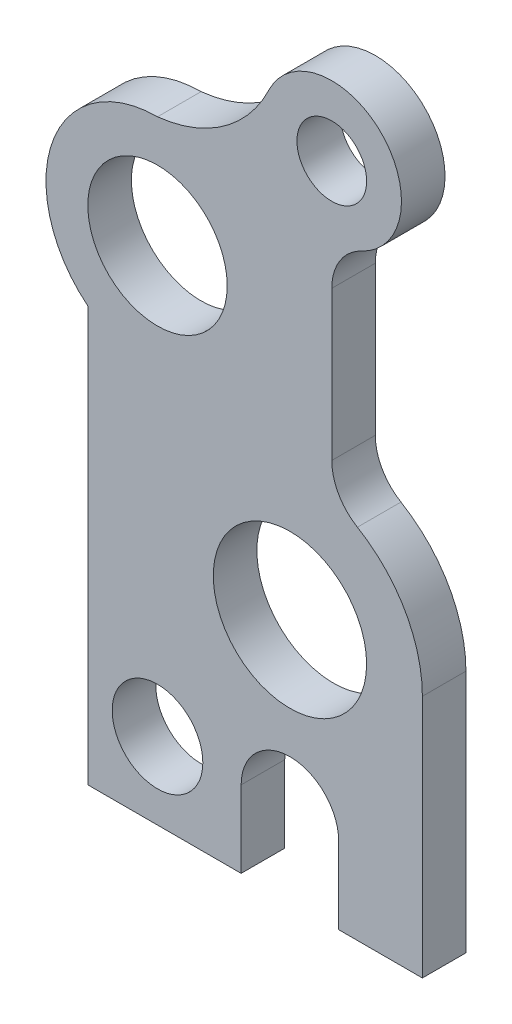
ISO-10303-21;
HEADER;
FILE_DESCRIPTION(('STEP AP214'),'2;1');
FILE_NAME('part.step','',(''),(''),'','','');
FILE_SCHEMA(('AUTOMOTIVE_DESIGN { 1 0 10303 214 1 1 1 1 }'));
ENDSEC;
DATA;
#1=APPLICATION_CONTEXT('core data for automotive mechanical design processes');
#2=APPLICATION_PROTOCOL_DEFINITION('international standard','automotive_design',2000,#1);
#3=PRODUCT_CONTEXT('',#1,'mechanical');
#4=PRODUCT('Part','Part','',(#3));
#5=PRODUCT_RELATED_PRODUCT_CATEGORY('part','',(#4));
#6=PRODUCT_DEFINITION_FORMATION('','',#4);
#7=PRODUCT_DEFINITION_CONTEXT('part definition',#1,'design');
#8=PRODUCT_DEFINITION('design','',#6,#7);
#9=PRODUCT_DEFINITION_SHAPE('','',#8);
#10=(LENGTH_UNIT() NAMED_UNIT(*) SI_UNIT(.MILLI.,.METRE.));
#11=(NAMED_UNIT(*) PLANE_ANGLE_UNIT() SI_UNIT($,.RADIAN.));
#12=(NAMED_UNIT(*) SI_UNIT($,.STERADIAN.) SOLID_ANGLE_UNIT());
#13=UNCERTAINTY_MEASURE_WITH_UNIT(LENGTH_MEASURE(1.E-05),#10,'distance_accuracy_value','');
#14=(GEOMETRIC_REPRESENTATION_CONTEXT(3) GLOBAL_UNCERTAINTY_ASSIGNED_CONTEXT((#13)) GLOBAL_UNIT_ASSIGNED_CONTEXT((#10,
#11,#12)) REPRESENTATION_CONTEXT('',''));
#15=CARTESIAN_POINT('',(0.,0.,0.));
#16=DIRECTION('',(0.,0.,1.));
#17=DIRECTION('',(1.,0.,0.));
#18=AXIS2_PLACEMENT_3D('',#15,#16,#17);
#19=CARTESIAN_POINT('',(96.,0.,12.5));
#20=DIRECTION('',(-1.,0.,0.));
#21=DIRECTION('',(0.,0.,1.));
#22=AXIS2_PLACEMENT_3D('',#19,#20,#21);
#23=PLANE('',#22);
#24=DIRECTION('',(0.,1.,0.));
#25=VECTOR('',#24,1.);
#26=CARTESIAN_POINT('',(96.,0.,0.));
#27=LINE('',#26,#25);
#28=CARTESIAN_POINT('',(96.,0.,0.));
#29=VERTEX_POINT('',#28);
#30=CARTESIAN_POINT('',(96.,70.,0.));
#31=VERTEX_POINT('',#30);
#32=EDGE_CURVE('E164',#29,#31,#27,.T.);
#33=ORIENTED_EDGE('',*,*,#32,.T.);
#34=DIRECTION('',(0.,0.,-1.));
#35=VECTOR('',#34,1.);
#36=CARTESIAN_POINT('',(96.,70.,12.5));
#37=LINE('',#36,#35);
#38=CARTESIAN_POINT('',(96.,70.,12.5));
#39=VERTEX_POINT('',#38);
#40=EDGE_CURVE('E144',#39,#31,#37,.T.);
#41=ORIENTED_EDGE('',*,*,#40,.F.);
#42=DIRECTION('',(0.,1.,0.));
#43=VECTOR('',#42,1.);
#44=CARTESIAN_POINT('',(96.,0.,12.5));
#45=LINE('',#44,#43);
#46=CARTESIAN_POINT('',(96.,0.,12.5));
#47=VERTEX_POINT('',#46);
#48=EDGE_CURVE('E155',#47,#39,#45,.T.);
#49=ORIENTED_EDGE('',*,*,#48,.F.);
#50=DIRECTION('',(0.,0.,-1.));
#51=VECTOR('',#50,1.);
#52=CARTESIAN_POINT('',(96.,0.,12.5));
#53=LINE('',#52,#51);
#54=EDGE_CURVE('E191',#47,#29,#53,.T.);
#55=ORIENTED_EDGE('',*,*,#54,.T.);
#56=EDGE_LOOP('',(#33,#41,#49,#55));
#57=FACE_BOUND('',#56,.T.);
#58=ADVANCED_FACE('F41',(#57),#23,.F.);
#59=CARTESIAN_POINT('',(58.,70.,12.5));
#60=DIRECTION('',(0.,0.,-1.));
#61=DIRECTION('',(-1.,0.,0.));
#62=AXIS2_PLACEMENT_3D('',#59,#60,#61);
#63=CYLINDRICAL_SURFACE('',#62,38.);
#64=CARTESIAN_POINT('',(58.,70.,0.));
#65=DIRECTION('',(0.,0.,1.));
#66=DIRECTION('',(1.,0.,0.));
#67=AXIS2_PLACEMENT_3D('',#64,#65,#66);
#68=CIRCLE('',#67,38.);
#69=CARTESIAN_POINT('',(77.3584905660377,102.699370682088,0.));
#70=VERTEX_POINT('',#69);
#71=EDGE_CURVE('E240',#31,#70,#68,.T.);
#72=ORIENTED_EDGE('',*,*,#71,.T.);
#73=DIRECTION('',(0.,0.,-1.));
#74=VECTOR('',#73,1.);
#75=CARTESIAN_POINT('',(77.3584905660377,102.699370682088,12.5));
#76=LINE('',#75,#74);
#77=CARTESIAN_POINT('',(77.3584905660377,102.699370682088,12.5));
#78=VERTEX_POINT('',#77);
#79=EDGE_CURVE('E150',#78,#70,#76,.T.);
#80=ORIENTED_EDGE('',*,*,#79,.F.);
#81=CARTESIAN_POINT('',(58.,70.,12.5));
#82=DIRECTION('',(0.,0.,1.));
#83=DIRECTION('',(1.,0.,0.));
#84=AXIS2_PLACEMENT_3D('',#81,#82,#83);
#85=CIRCLE('',#84,38.);
#86=EDGE_CURVE('E136',#39,#78,#85,.T.);
#87=ORIENTED_EDGE('',*,*,#86,.F.);
#88=ORIENTED_EDGE('',*,*,#40,.T.);
#89=EDGE_LOOP('',(#72,#80,#87,#88));
#90=FACE_BOUND('',#89,.T.);
#91=ADVANCED_FACE('F141',(#90),#63,.T.);
#92=CARTESIAN_POINT('',(85.,115.607017003966,12.5));
#93=DIRECTION('',(0.,0.,-1.));
#94=DIRECTION('',(-1.,0.,0.));
#95=AXIS2_PLACEMENT_3D('',#92,#93,#94);
#96=CYLINDRICAL_SURFACE('',#95,15.);
#97=CARTESIAN_POINT('',(85.,115.607017003966,0.));
#98=DIRECTION('',(0.,0.,1.));
#99=DIRECTION('',(1.,0.,0.));
#100=AXIS2_PLACEMENT_3D('',#97,#98,#99);
#101=CIRCLE('',#100,15.);
#102=CARTESIAN_POINT('',(70.,115.607017003966,0.));
#103=VERTEX_POINT('',#102);
#104=EDGE_CURVE('E235',#103,#70,#101,.T.);
#105=ORIENTED_EDGE('',*,*,#104,.F.);
#106=DIRECTION('',(0.,0.,-1.));
#107=VECTOR('',#106,1.);
#108=CARTESIAN_POINT('',(70.,115.607017003966,12.5));
#109=LINE('',#108,#107);
#110=CARTESIAN_POINT('',(70.,115.607017003966,12.5));
#111=VERTEX_POINT('',#110);
#112=EDGE_CURVE('E168',#111,#103,#109,.T.);
#113=ORIENTED_EDGE('',*,*,#112,.F.);
#114=CARTESIAN_POINT('',(85.,115.607017003966,12.5));
#115=DIRECTION('',(0.,0.,1.));
#116=DIRECTION('',(1.,0.,0.));
#117=AXIS2_PLACEMENT_3D('',#114,#115,#116);
#118=CIRCLE('',#117,15.);
#119=EDGE_CURVE('E151',#111,#78,#118,.T.);
#120=ORIENTED_EDGE('',*,*,#119,.T.);
#121=ORIENTED_EDGE('',*,*,#79,.T.);
#122=EDGE_LOOP('',(#105,#113,#120,#121));
#123=FACE_BOUND('',#122,.T.);
#124=ADVANCED_FACE('F277',(#123),#96,.F.);
#125=CARTESIAN_POINT('',(70.,0.,12.5));
#126=DIRECTION('',(1.,0.,0.));
#127=DIRECTION('',(0.,0.,-1.));
#128=AXIS2_PLACEMENT_3D('',#125,#126,#127);
#129=PLANE('',#128);
#130=DIRECTION('',(0.,-1.,0.));
#131=VECTOR('',#130,1.);
#132=CARTESIAN_POINT('',(70.,0.,0.));
#133=LINE('',#132,#131);
#134=CARTESIAN_POINT('',(70.,158.377223398316,0.));
#135=VERTEX_POINT('',#134);
#136=EDGE_CURVE('E234',#135,#103,#133,.T.);
#137=ORIENTED_EDGE('',*,*,#136,.F.);
#138=DIRECTION('',(0.,0.,-1.));
#139=VECTOR('',#138,1.);
#140=CARTESIAN_POINT('',(70.,158.377223398316,12.5));
#141=LINE('',#140,#139);
#142=CARTESIAN_POINT('',(70.,158.377223398316,12.5));
#143=VERTEX_POINT('',#142);
#144=EDGE_CURVE('E57',#135,#143,#141,.F.);
#145=ORIENTED_EDGE('',*,*,#144,.T.);
#146=DIRECTION('',(0.,-1.,0.));
#147=VECTOR('',#146,1.);
#148=CARTESIAN_POINT('',(70.,0.,12.5));
#149=LINE('',#148,#147);
#150=EDGE_CURVE('E271',#143,#111,#149,.T.);
#151=ORIENTED_EDGE('',*,*,#150,.T.);
#152=ORIENTED_EDGE('',*,*,#112,.T.);
#153=EDGE_LOOP('',(#137,#145,#151,#152));
#154=FACE_BOUND('',#153,.T.);
#155=ADVANCED_FACE('F321',(#154),#129,.T.);
#156=CARTESIAN_POINT('',(70.,190.,12.5));
#157=DIRECTION('',(0.,0.,-1.));
#158=DIRECTION('',(-1.,0.,0.));
#159=AXIS2_PLACEMENT_3D('',#156,#157,#158);
#160=CYLINDRICAL_SURFACE('',#159,20.);
#161=CARTESIAN_POINT('',(70.,190.,12.5));
#162=DIRECTION('',(0.,0.,1.));
#163=DIRECTION('',(1.,0.,0.));
#164=AXIS2_PLACEMENT_3D('',#161,#162,#163);
#165=CIRCLE('',#164,20.);
#166=CARTESIAN_POINT('',(78.5714285714286,171.929841941895,12.5));
#167=VERTEX_POINT('',#166);
#168=CARTESIAN_POINT('',(51.9999999999999,198.717797887081,12.5));
#169=VERTEX_POINT('',#168);
#170=EDGE_CURVE('E267',#167,#169,#165,.T.);
#171=ORIENTED_EDGE('',*,*,#170,.F.);
#172=DIRECTION('',(0.,0.,-1.));
#173=VECTOR('',#172,1.);
#174=CARTESIAN_POINT('',(78.5714285714286,171.929841941895,12.5));
#175=LINE('',#174,#173);
#176=CARTESIAN_POINT('',(78.5714285714286,171.929841941895,0.));
#177=VERTEX_POINT('',#176);
#178=EDGE_CURVE('E167',#167,#177,#175,.T.);
#179=ORIENTED_EDGE('',*,*,#178,.T.);
#180=CARTESIAN_POINT('',(70.,190.,0.));
#181=DIRECTION('',(0.,0.,1.));
#182=DIRECTION('',(1.,0.,0.));
#183=AXIS2_PLACEMENT_3D('',#180,#181,#182);
#184=CIRCLE('',#183,20.);
#185=CARTESIAN_POINT('',(51.9999999999999,198.717797887081,0.));
#186=VERTEX_POINT('',#185);
#187=EDGE_CURVE('E227',#177,#186,#184,.T.);
#188=ORIENTED_EDGE('',*,*,#187,.T.);
#189=DIRECTION('',(0.,0.,-1.));
#190=VECTOR('',#189,1.);
#191=CARTESIAN_POINT('',(51.9999999999999,198.717797887081,12.5));
#192=LINE('',#191,#190);
#193=EDGE_CURVE('E178',#169,#186,#192,.T.);
#194=ORIENTED_EDGE('',*,*,#193,.F.);
#195=EDGE_LOOP('',(#171,#179,#188,#194));
#196=FACE_BOUND('',#195,.T.);
#197=ADVANCED_FACE('F285',(#196),#160,.T.);
#198=CARTESIAN_POINT('',(15.8221100087037,215.781217115878,12.5));
#199=DIRECTION('',(0.,0.,-1.));
#200=DIRECTION('',(-1.,0.,0.));
#201=AXIS2_PLACEMENT_3D('',#198,#199,#200);
#202=CYLINDRICAL_SURFACE('',#201,40.);
#203=CARTESIAN_POINT('',(15.8221100087037,215.781217115878,0.));
#204=DIRECTION('',(0.,0.,1.));
#205=DIRECTION('',(1.,0.,0.));
#206=AXIS2_PLACEMENT_3D('',#203,#204,#205);
#207=CIRCLE('',#206,40.);
#208=CARTESIAN_POINT('',(20.,176.,0.));
#209=VERTEX_POINT('',#208);
#210=EDGE_CURVE('E226',#186,#209,#207,.F.);
#211=ORIENTED_EDGE('',*,*,#210,.T.);
#212=DIRECTION('',(0.,0.,-1.));
#213=VECTOR('',#212,1.);
#214=CARTESIAN_POINT('',(20.,176.,12.5));
#215=LINE('',#214,#213);
#216=CARTESIAN_POINT('',(20.,176.,12.5));
#217=VERTEX_POINT('',#216);
#218=EDGE_CURVE('E180',#217,#209,#215,.T.);
#219=ORIENTED_EDGE('',*,*,#218,.F.);
#220=CARTESIAN_POINT('',(15.8221100087037,215.781217115878,12.5));
#221=DIRECTION('',(0.,0.,1.));
#222=DIRECTION('',(1.,0.,0.));
#223=AXIS2_PLACEMENT_3D('',#220,#221,#222);
#224=CIRCLE('',#223,40.);
#225=EDGE_CURVE('E270',#169,#217,#224,.F.);
#226=ORIENTED_EDGE('',*,*,#225,.F.);
#227=ORIENTED_EDGE('',*,*,#193,.T.);
#228=EDGE_LOOP('',(#211,#219,#226,#227));
#229=FACE_BOUND('',#228,.T.);
#230=ADVANCED_FACE('F286',(#229),#202,.F.);
#231=CARTESIAN_POINT('',(20.,144.,12.5));
#232=DIRECTION('',(0.,0.,-1.));
#233=DIRECTION('',(-1.,0.,0.));
#234=AXIS2_PLACEMENT_3D('',#231,#232,#233);
#235=CYLINDRICAL_SURFACE('',#234,32.);
#236=CARTESIAN_POINT('',(20.,144.,0.));
#237=DIRECTION('',(0.,0.,1.));
#238=DIRECTION('',(1.,0.,0.));
#239=AXIS2_PLACEMENT_3D('',#236,#237,#238);
#240=CIRCLE('',#239,32.);
#241=CARTESIAN_POINT('',(0.,119.020008006406,0.));
#242=VERTEX_POINT('',#241);
#243=EDGE_CURVE('E223',#209,#242,#240,.T.);
#244=ORIENTED_EDGE('',*,*,#243,.T.);
#245=DIRECTION('',(0.,0.,-1.));
#246=VECTOR('',#245,1.);
#247=CARTESIAN_POINT('',(0.,119.020008006406,12.5));
#248=LINE('',#247,#246);
#249=CARTESIAN_POINT('',(0.,119.020008006406,12.5));
#250=VERTEX_POINT('',#249);
#251=EDGE_CURVE('E185',#250,#242,#248,.T.);
#252=ORIENTED_EDGE('',*,*,#251,.F.);
#253=CARTESIAN_POINT('',(20.,144.,12.5));
#254=DIRECTION('',(0.,0.,1.));
#255=DIRECTION('',(1.,0.,0.));
#256=AXIS2_PLACEMENT_3D('',#253,#254,#255);
#257=CIRCLE('',#256,32.);
#258=EDGE_CURVE('E264',#217,#250,#257,.T.);
#259=ORIENTED_EDGE('',*,*,#258,.F.);
#260=ORIENTED_EDGE('',*,*,#218,.T.);
#261=EDGE_LOOP('',(#244,#252,#259,#260));
#262=FACE_BOUND('',#261,.T.);
#263=ADVANCED_FACE('F294',(#262),#235,.T.);
#264=CARTESIAN_POINT('',(0.,0.,12.5));
#265=DIRECTION('',(-1.,0.,0.));
#266=DIRECTION('',(0.,0.,1.));
#267=AXIS2_PLACEMENT_3D('',#264,#265,#266);
#268=PLANE('',#267);
#269=DIRECTION('',(0.,1.,0.));
#270=VECTOR('',#269,1.);
#271=CARTESIAN_POINT('',(0.,0.,0.));
#272=LINE('',#271,#270);
#273=CARTESIAN_POINT('',(0.,0.,0.));
#274=VERTEX_POINT('',#273);
#275=EDGE_CURVE('E225',#274,#242,#272,.T.);
#276=ORIENTED_EDGE('',*,*,#275,.F.);
#277=DIRECTION('',(0.,0.,-1.));
#278=VECTOR('',#277,1.);
#279=CARTESIAN_POINT('',(0.,0.,12.5));
#280=LINE('',#279,#278);
#281=CARTESIAN_POINT('',(0.,0.,12.5));
#282=VERTEX_POINT('',#281);
#283=EDGE_CURVE('E184',#282,#274,#280,.T.);
#284=ORIENTED_EDGE('',*,*,#283,.F.);
#285=DIRECTION('',(0.,1.,0.));
#286=VECTOR('',#285,1.);
#287=CARTESIAN_POINT('',(0.,0.,12.5));
#288=LINE('',#287,#286);
#289=EDGE_CURVE('E265',#282,#250,#288,.T.);
#290=ORIENTED_EDGE('',*,*,#289,.T.);
#291=ORIENTED_EDGE('',*,*,#251,.T.);
#292=EDGE_LOOP('',(#276,#284,#290,#291));
#293=FACE_BOUND('',#292,.T.);
#294=ADVANCED_FACE('F304',(#293),#268,.T.);
#295=CARTESIAN_POINT('',(0.,0.,12.5));
#296=DIRECTION('',(0.,1.,0.));
#297=DIRECTION('',(0.,0.,1.));
#298=AXIS2_PLACEMENT_3D('',#295,#296,#297);
#299=PLANE('',#298);
#300=DIRECTION('',(1.,0.,0.));
#301=VECTOR('',#300,1.);
#302=CARTESIAN_POINT('',(0.,0.,0.));
#303=LINE('',#302,#301);
#304=CARTESIAN_POINT('',(44.,0.,0.));
#305=VERTEX_POINT('',#304);
#306=EDGE_CURVE('E218',#274,#305,#303,.T.);
#307=ORIENTED_EDGE('',*,*,#306,.T.);
#308=DIRECTION('',(0.,0.,-1.));
#309=VECTOR('',#308,1.);
#310=CARTESIAN_POINT('',(44.,0.,12.5));
#311=LINE('',#310,#309);
#312=CARTESIAN_POINT('',(44.,0.,12.5));
#313=VERTEX_POINT('',#312);
#314=EDGE_CURVE('E188',#313,#305,#311,.T.);
#315=ORIENTED_EDGE('',*,*,#314,.F.);
#316=DIRECTION('',(1.,0.,0.));
#317=VECTOR('',#316,1.);
#318=CARTESIAN_POINT('',(0.,0.,12.5));
#319=LINE('',#318,#317);
#320=EDGE_CURVE('E257',#282,#313,#319,.T.);
#321=ORIENTED_EDGE('',*,*,#320,.F.);
#322=ORIENTED_EDGE('',*,*,#283,.T.);
#323=EDGE_LOOP('',(#307,#315,#321,#322));
#324=FACE_BOUND('',#323,.T.);
#325=ADVANCED_FACE('F301',(#324),#299,.F.);
#326=CARTESIAN_POINT('',(44.,0.,12.5));
#327=DIRECTION('',(1.,0.,0.));
#328=DIRECTION('',(0.,0.,-1.));
#329=AXIS2_PLACEMENT_3D('',#326,#327,#328);
#330=PLANE('',#329);
#331=DIRECTION('',(0.,-1.,0.));
#332=VECTOR('',#331,1.);
#333=CARTESIAN_POINT('',(44.,0.,0.));
#334=LINE('',#333,#332);
#335=CARTESIAN_POINT('',(44.,22.,0.));
#336=VERTEX_POINT('',#335);
#337=EDGE_CURVE('E216',#336,#305,#334,.T.);
#338=ORIENTED_EDGE('',*,*,#337,.F.);
#339=DIRECTION('',(0.,0.,-1.));
#340=VECTOR('',#339,1.);
#341=CARTESIAN_POINT('',(44.,22.,12.5));
#342=LINE('',#341,#340);
#343=CARTESIAN_POINT('',(44.,22.,12.5));
#344=VERTEX_POINT('',#343);
#345=EDGE_CURVE('E186',#344,#336,#342,.T.);
#346=ORIENTED_EDGE('',*,*,#345,.F.);
#347=DIRECTION('',(0.,-1.,0.));
#348=VECTOR('',#347,1.);
#349=CARTESIAN_POINT('',(44.,0.,12.5));
#350=LINE('',#349,#348);
#351=EDGE_CURVE('E260',#344,#313,#350,.T.);
#352=ORIENTED_EDGE('',*,*,#351,.T.);
#353=ORIENTED_EDGE('',*,*,#314,.T.);
#354=EDGE_LOOP('',(#338,#346,#352,#353));
#355=FACE_BOUND('',#354,.T.);
#356=ADVANCED_FACE('F306',(#355),#330,.T.);
#357=CARTESIAN_POINT('',(58.,22.,12.5));
#358=DIRECTION('',(0.,0.,-1.));
#359=DIRECTION('',(-1.,0.,0.));
#360=AXIS2_PLACEMENT_3D('',#357,#358,#359);
#361=CYLINDRICAL_SURFACE('',#360,14.);
#362=CARTESIAN_POINT('',(58.,22.,0.));
#363=DIRECTION('',(0.,0.,1.));
#364=DIRECTION('',(1.,0.,0.));
#365=AXIS2_PLACEMENT_3D('',#362,#363,#364);
#366=CIRCLE('',#365,14.);
#367=CARTESIAN_POINT('',(72.,22.,0.));
#368=VERTEX_POINT('',#367);
#369=EDGE_CURVE('E213',#368,#336,#366,.T.);
#370=ORIENTED_EDGE('',*,*,#369,.F.);
#371=DIRECTION('',(0.,0.,-1.));
#372=VECTOR('',#371,1.);
#373=CARTESIAN_POINT('',(72.,22.,12.5));
#374=LINE('',#373,#372);
#375=CARTESIAN_POINT('',(72.,22.,12.5));
#376=VERTEX_POINT('',#375);
#377=EDGE_CURVE('E187',#376,#368,#374,.T.);
#378=ORIENTED_EDGE('',*,*,#377,.F.);
#379=CARTESIAN_POINT('',(58.,22.,12.5));
#380=DIRECTION('',(0.,0.,1.));
#381=DIRECTION('',(1.,0.,0.));
#382=AXIS2_PLACEMENT_3D('',#379,#380,#381);
#383=CIRCLE('',#382,14.);
#384=EDGE_CURVE('E255',#376,#344,#383,.T.);
#385=ORIENTED_EDGE('',*,*,#384,.T.);
#386=ORIENTED_EDGE('',*,*,#345,.T.);
#387=EDGE_LOOP('',(#370,#378,#385,#386));
#388=FACE_BOUND('',#387,.T.);
#389=ADVANCED_FACE('F315',(#388),#361,.F.);
#390=CARTESIAN_POINT('',(72.,0.,12.5));
#391=DIRECTION('',(1.,0.,0.));
#392=DIRECTION('',(0.,0.,-1.));
#393=AXIS2_PLACEMENT_3D('',#390,#391,#392);
#394=PLANE('',#393);
#395=DIRECTION('',(0.,-1.,0.));
#396=VECTOR('',#395,1.);
#397=CARTESIAN_POINT('',(72.,0.,0.));
#398=LINE('',#397,#396);
#399=CARTESIAN_POINT('',(72.,0.,0.));
#400=VERTEX_POINT('',#399);
#401=EDGE_CURVE('E211',#368,#400,#398,.T.);
#402=ORIENTED_EDGE('',*,*,#401,.T.);
#403=DIRECTION('',(0.,0.,-1.));
#404=VECTOR('',#403,1.);
#405=CARTESIAN_POINT('',(72.,0.,12.5));
#406=LINE('',#405,#404);
#407=CARTESIAN_POINT('',(72.,0.,12.5));
#408=VERTEX_POINT('',#407);
#409=EDGE_CURVE('E194',#408,#400,#406,.T.);
#410=ORIENTED_EDGE('',*,*,#409,.F.);
#411=DIRECTION('',(0.,-1.,0.));
#412=VECTOR('',#411,1.);
#413=CARTESIAN_POINT('',(72.,0.,12.5));
#414=LINE('',#413,#412);
#415=EDGE_CURVE('E252',#376,#408,#414,.T.);
#416=ORIENTED_EDGE('',*,*,#415,.F.);
#417=ORIENTED_EDGE('',*,*,#377,.T.);
#418=EDGE_LOOP('',(#402,#410,#416,#417));
#419=FACE_BOUND('',#418,.T.);
#420=ADVANCED_FACE('F320',(#419),#394,.F.);
#421=CARTESIAN_POINT('',(20.,144.,12.5));
#422=DIRECTION('',(0.,0.,-1.));
#423=DIRECTION('',(-1.,0.,0.));
#424=AXIS2_PLACEMENT_3D('',#421,#422,#423);
#425=CYLINDRICAL_SURFACE('',#424,20.);
#426=CARTESIAN_POINT('',(20.,144.,12.5));
#427=DIRECTION('',(0.,0.,1.));
#428=DIRECTION('',(1.,0.,0.));
#429=AXIS2_PLACEMENT_3D('',#426,#427,#428);
#430=CIRCLE('',#429,20.);
#431=CARTESIAN_POINT('',(40.,144.,12.5));
#432=VERTEX_POINT('',#431);
#433=EDGE_CURVE('E245',#432,#432,#430,.T.);
#434=ORIENTED_EDGE('',*,*,#433,.T.);
#435=EDGE_LOOP('',(#434));
#436=FACE_BOUND('',#435,.T.);
#437=CARTESIAN_POINT('',(20.,144.,0.));
#438=DIRECTION('',(0.,0.,1.));
#439=DIRECTION('',(1.,0.,0.));
#440=AXIS2_PLACEMENT_3D('',#437,#438,#439);
#441=CIRCLE('',#440,20.);
#442=CARTESIAN_POINT('',(40.,144.,0.));
#443=VERTEX_POINT('',#442);
#444=EDGE_CURVE('E199',#443,#443,#441,.T.);
#445=ORIENTED_EDGE('',*,*,#444,.F.);
#446=EDGE_LOOP('',(#445));
#447=FACE_BOUND('',#446,.T.);
#448=ADVANCED_FACE('F391',(#436,#447),#425,.F.);
#449=CARTESIAN_POINT('',(58.,70.,12.5));
#450=DIRECTION('',(0.,0.,-1.));
#451=DIRECTION('',(-1.,0.,0.));
#452=AXIS2_PLACEMENT_3D('',#449,#450,#451);
#453=CYLINDRICAL_SURFACE('',#452,22.);
#454=CARTESIAN_POINT('',(58.,70.,12.5));
#455=DIRECTION('',(0.,0.,1.));
#456=DIRECTION('',(1.,0.,0.));
#457=AXIS2_PLACEMENT_3D('',#454,#455,#456);
#458=CIRCLE('',#457,22.);
#459=CARTESIAN_POINT('',(80.,70.,12.5));
#460=VERTEX_POINT('',#459);
#461=EDGE_CURVE('E242',#460,#460,#458,.T.);
#462=ORIENTED_EDGE('',*,*,#461,.T.);
#463=EDGE_LOOP('',(#462));
#464=FACE_BOUND('',#463,.T.);
#465=CARTESIAN_POINT('',(58.,70.,0.));
#466=DIRECTION('',(0.,0.,1.));
#467=DIRECTION('',(1.,0.,0.));
#468=AXIS2_PLACEMENT_3D('',#465,#466,#467);
#469=CIRCLE('',#468,22.);
#470=CARTESIAN_POINT('',(80.,70.,0.));
#471=VERTEX_POINT('',#470);
#472=EDGE_CURVE('E201',#471,#471,#469,.T.);
#473=ORIENTED_EDGE('',*,*,#472,.F.);
#474=EDGE_LOOP('',(#473));
#475=FACE_BOUND('',#474,.T.);
#476=ADVANCED_FACE('F402',(#464,#475),#453,.F.);
#477=CARTESIAN_POINT('',(20.,22.,12.5));
#478=DIRECTION('',(0.,0.,-1.));
#479=DIRECTION('',(-1.,0.,0.));
#480=AXIS2_PLACEMENT_3D('',#477,#478,#479);
#481=CYLINDRICAL_SURFACE('',#480,13.);
#482=CARTESIAN_POINT('',(20.,22.,12.5));
#483=DIRECTION('',(0.,0.,1.));
#484=DIRECTION('',(1.,0.,0.));
#485=AXIS2_PLACEMENT_3D('',#482,#483,#484);
#486=CIRCLE('',#485,13.);
#487=CARTESIAN_POINT('',(33.,22.,12.5));
#488=VERTEX_POINT('',#487);
#489=EDGE_CURVE('E247',#488,#488,#486,.T.);
#490=ORIENTED_EDGE('',*,*,#489,.T.);
#491=EDGE_LOOP('',(#490));
#492=FACE_BOUND('',#491,.T.);
#493=CARTESIAN_POINT('',(20.,22.,0.));
#494=DIRECTION('',(0.,0.,1.));
#495=DIRECTION('',(1.,0.,0.));
#496=AXIS2_PLACEMENT_3D('',#493,#494,#495);
#497=CIRCLE('',#496,13.);
#498=CARTESIAN_POINT('',(33.,22.,0.));
#499=VERTEX_POINT('',#498);
#500=EDGE_CURVE('E206',#499,#499,#497,.T.);
#501=ORIENTED_EDGE('',*,*,#500,.F.);
#502=EDGE_LOOP('',(#501));
#503=FACE_BOUND('',#502,.T.);
#504=ADVANCED_FACE('F407',(#492,#503),#481,.F.);
#505=CARTESIAN_POINT('',(0.,0.,12.5));
#506=DIRECTION('',(0.,1.,0.));
#507=DIRECTION('',(0.,0.,1.));
#508=AXIS2_PLACEMENT_3D('',#505,#506,#507);
#509=PLANE('',#508);
#510=DIRECTION('',(1.,0.,0.));
#511=VECTOR('',#510,1.);
#512=CARTESIAN_POINT('',(0.,0.,0.));
#513=LINE('',#512,#511);
#514=EDGE_CURVE('E207',#400,#29,#513,.T.);
#515=ORIENTED_EDGE('',*,*,#514,.T.);
#516=ORIENTED_EDGE('',*,*,#54,.F.);
#517=DIRECTION('',(1.,0.,0.));
#518=VECTOR('',#517,1.);
#519=CARTESIAN_POINT('',(0.,0.,12.5));
#520=LINE('',#519,#518);
#521=EDGE_CURVE('E158',#408,#47,#520,.T.);
#522=ORIENTED_EDGE('',*,*,#521,.F.);
#523=ORIENTED_EDGE('',*,*,#409,.T.);
#524=EDGE_LOOP('',(#515,#516,#522,#523));
#525=FACE_BOUND('',#524,.T.);
#526=ADVANCED_FACE('F319',(#525),#509,.F.);
#527=CARTESIAN_POINT('',(70.,190.,12.5));
#528=DIRECTION('',(0.,0.,-1.));
#529=DIRECTION('',(-1.,0.,0.));
#530=AXIS2_PLACEMENT_3D('',#527,#528,#529);
#531=CYLINDRICAL_SURFACE('',#530,10.);
#532=CARTESIAN_POINT('',(70.,190.,12.5));
#533=DIRECTION('',(0.,0.,1.));
#534=DIRECTION('',(1.,0.,0.));
#535=AXIS2_PLACEMENT_3D('',#532,#533,#534);
#536=CIRCLE('',#535,10.);
#537=CARTESIAN_POINT('',(80.,190.,12.5));
#538=VERTEX_POINT('',#537);
#539=EDGE_CURVE('E197',#538,#538,#536,.T.);
#540=ORIENTED_EDGE('',*,*,#539,.T.);
#541=EDGE_LOOP('',(#540));
#542=FACE_BOUND('',#541,.T.);
#543=CARTESIAN_POINT('',(70.,190.,0.));
#544=DIRECTION('',(0.,0.,1.));
#545=DIRECTION('',(1.,0.,0.));
#546=AXIS2_PLACEMENT_3D('',#543,#544,#545);
#547=CIRCLE('',#546,10.);
#548=CARTESIAN_POINT('',(80.,190.,0.));
#549=VERTEX_POINT('',#548);
#550=EDGE_CURVE('E165',#549,#549,#547,.T.);
#551=ORIENTED_EDGE('',*,*,#550,.F.);
#552=EDGE_LOOP('',(#551));
#553=FACE_BOUND('',#552,.T.);
#554=ADVANCED_FACE('F426',(#542,#553),#531,.F.);
#555=CARTESIAN_POINT('',(0.,0.,12.5));
#556=DIRECTION('',(0.,0.,1.));
#557=DIRECTION('',(1.,0.,0.));
#558=AXIS2_PLACEMENT_3D('',#555,#556,#557);
#559=PLANE('',#558);
#560=ORIENTED_EDGE('',*,*,#48,.T.);
#561=ORIENTED_EDGE('',*,*,#86,.T.);
#562=ORIENTED_EDGE('',*,*,#119,.F.);
#563=ORIENTED_EDGE('',*,*,#150,.F.);
#564=CARTESIAN_POINT('',(85.,158.377223398316,12.5));
#565=DIRECTION('',(0.,0.,1.));
#566=DIRECTION('',(1.,0.,0.));
#567=AXIS2_PLACEMENT_3D('',#564,#565,#566);
#568=CIRCLE('',#567,15.);
#569=EDGE_CURVE('E11',#143,#167,#568,.F.);
#570=ORIENTED_EDGE('',*,*,#569,.T.);
#571=ORIENTED_EDGE('',*,*,#170,.T.);
#572=ORIENTED_EDGE('',*,*,#225,.T.);
#573=ORIENTED_EDGE('',*,*,#258,.T.);
#574=ORIENTED_EDGE('',*,*,#289,.F.);
#575=ORIENTED_EDGE('',*,*,#320,.T.);
#576=ORIENTED_EDGE('',*,*,#351,.F.);
#577=ORIENTED_EDGE('',*,*,#384,.F.);
#578=ORIENTED_EDGE('',*,*,#415,.T.);
#579=ORIENTED_EDGE('',*,*,#521,.T.);
#580=EDGE_LOOP('',(#560,#561,#562,#563,#570,#571,#572,#573,#574,#575,#576,#577,#578,#579));
#581=FACE_BOUND('',#580,.T.);
#582=ORIENTED_EDGE('',*,*,#489,.F.);
#583=EDGE_LOOP('',(#582));
#584=FACE_BOUND('',#583,.T.);
#585=ORIENTED_EDGE('',*,*,#461,.F.);
#586=EDGE_LOOP('',(#585));
#587=FACE_BOUND('',#586,.T.);
#588=ORIENTED_EDGE('',*,*,#433,.F.);
#589=EDGE_LOOP('',(#588));
#590=FACE_BOUND('',#589,.T.);
#591=ORIENTED_EDGE('',*,*,#539,.F.);
#592=EDGE_LOOP('',(#591));
#593=FACE_BOUND('',#592,.T.);
#594=ADVANCED_FACE('F154',(#581,#584,#587,#590,#593),#559,.T.);
#595=CARTESIAN_POINT('',(0.,0.,0.));
#596=DIRECTION('',(0.,0.,1.));
#597=DIRECTION('',(1.,0.,0.));
#598=AXIS2_PLACEMENT_3D('',#595,#596,#597);
#599=PLANE('',#598);
#600=ORIENTED_EDGE('',*,*,#32,.F.);
#601=ORIENTED_EDGE('',*,*,#514,.F.);
#602=ORIENTED_EDGE('',*,*,#401,.F.);
#603=ORIENTED_EDGE('',*,*,#369,.T.);
#604=ORIENTED_EDGE('',*,*,#337,.T.);
#605=ORIENTED_EDGE('',*,*,#306,.F.);
#606=ORIENTED_EDGE('',*,*,#275,.T.);
#607=ORIENTED_EDGE('',*,*,#243,.F.);
#608=ORIENTED_EDGE('',*,*,#210,.F.);
#609=ORIENTED_EDGE('',*,*,#187,.F.);
#610=CARTESIAN_POINT('',(85.,158.377223398316,0.));
#611=DIRECTION('',(0.,0.,1.));
#612=DIRECTION('',(1.,0.,0.));
#613=AXIS2_PLACEMENT_3D('',#610,#611,#612);
#614=CIRCLE('',#613,15.);
#615=EDGE_CURVE('E47',#177,#135,#614,.T.);
#616=ORIENTED_EDGE('',*,*,#615,.T.);
#617=ORIENTED_EDGE('',*,*,#136,.T.);
#618=ORIENTED_EDGE('',*,*,#104,.T.);
#619=ORIENTED_EDGE('',*,*,#71,.F.);
#620=EDGE_LOOP('',(#600,#601,#602,#603,#604,#605,#606,#607,#608,#609,#616,#617,#618,#619));
#621=FACE_BOUND('',#620,.T.);
#622=ORIENTED_EDGE('',*,*,#500,.T.);
#623=EDGE_LOOP('',(#622));
#624=FACE_BOUND('',#623,.T.);
#625=ORIENTED_EDGE('',*,*,#472,.T.);
#626=EDGE_LOOP('',(#625));
#627=FACE_BOUND('',#626,.T.);
#628=ORIENTED_EDGE('',*,*,#444,.T.);
#629=EDGE_LOOP('',(#628));
#630=FACE_BOUND('',#629,.T.);
#631=ORIENTED_EDGE('',*,*,#550,.T.);
#632=EDGE_LOOP('',(#631));
#633=FACE_BOUND('',#632,.T.);
#634=ADVANCED_FACE('F282',(#621,#624,#627,#630,#633),#599,.F.);
#635=CARTESIAN_POINT('',(85.,158.377223398316,12.5));
#636=DIRECTION('',(0.,0.,-1.));
#637=DIRECTION('',(-1.,0.,0.));
#638=AXIS2_PLACEMENT_3D('',#635,#636,#637);
#639=CYLINDRICAL_SURFACE('',#638,15.);
#640=ORIENTED_EDGE('',*,*,#569,.F.);
#641=ORIENTED_EDGE('',*,*,#144,.F.);
#642=ORIENTED_EDGE('',*,*,#615,.F.);
#643=ORIENTED_EDGE('',*,*,#178,.F.);
#644=EDGE_LOOP('',(#640,#641,#642,#643));
#645=FACE_BOUND('',#644,.T.);
#646=ADVANCED_FACE('F43',(#645),#639,.F.);
#647=CLOSED_SHELL('',(#58,#91,#124,#155,#197,#230,#263,#294,#325,#356,#389,#420,#448,#476,#504,
#526,#554,#594,#634,#646));
#648=MANIFOLD_SOLID_BREP('B2',#647);
#649=ADVANCED_BREP_SHAPE_REPRESENTATION('',(#18,#648),#14);
#650=SHAPE_DEFINITION_REPRESENTATION(#9,#649);
ENDSEC;
END-ISO-10303-21;
